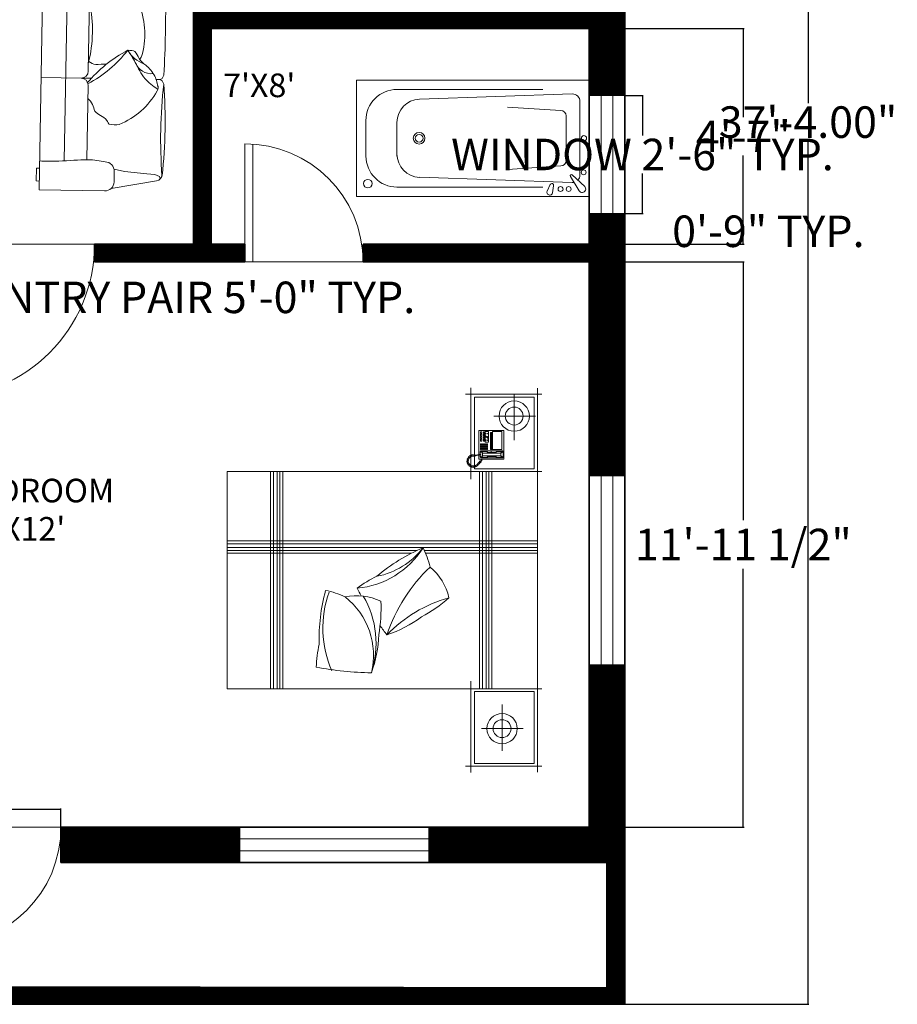
# Model space of a CAD drawing. Units: inches. Extents: x 108 to 771, y 58 to 590.
# Tile 7 of 8: x 524 to 747, y 100 to 350. Entities that reach past the tile are written whole.
import ezdxf

# ---------------------------------------------------------------- set-up
doc = ezdxf.new("R2010")
doc.units = ezdxf.units.IN
doc.header["$MEASUREMENT"] = 0
for name, color, linetype, lineweight in [('A-ANNO-DIMS', 2, 'Continuous', 13), ('A-AREA-IDEN', 7, 'Continuous', 18), ('A-DOOR', 3, 'Continuous', 18), ('A-FLOR-FIXT', 8, 'Continuous', 15), ('A-GLAZ', 4, 'Continuous', 18), ('A-WALL', 7, 'Continuous', 35), ('A-WALL-PATT', 252, 'Continuous', 9), ('Furniture', 7, 'Continuous', 15)]:
    doc.layers.add(name, color=color, linetype=linetype, lineweight=lineweight)
doc.styles.get("Standard").update_dxf_attribs({"font": 'italic8.shx'})
doc.dimstyles.get("Standard").update_dxf_attribs({"dimtxt": 8, "dimasz": 0.18, "dimexe": 0.18, "dimexo": 0.0625, "dimgap": 0.09, "dimtad": 0, "dimtih": 1, "dimtoh": 1, "dimzin": 0, "dimdsep": 46, "dimlunit": 3, "dimtxsty": 'Standard', "dimcen": 0.09, "dimclrt": 6, "dimadec": 0, "dimazin": 0, "dimtfac": 1, "dimtofl": 0, "dimtmove": 0, "dimatfit": 3, "dimfxl": 1, "dimtolj": 1, "dimtzin": 0, "dimarcsym": 0})

# ---------------------------------------------------------------- blocks, each defined once
blk = doc.blocks.new('*D6')
at = {"layer": 'A-ANNO-DIMS', "color": 0, "lineweight": -2, "transparency": 16777216}
for p, q in [((677.41, 548.05), (724.06, 548.05)), ((723.88, 547.87), (723.88, 328.9)), ((723.88, 100.23), (723.88, 319.2)), ((677.41, 100.05), (724.06, 100.05))]:
    blk.add_line(p, q, dxfattribs=at)
at = {"layer": 'A-ANNO-DIMS', "color": 0, "transparency": 16777216}
for points in [[(723.85, 547.87), (723.91, 547.87), (723.88, 548.05)], [(723.85, 100.23), (723.91, 100.23), (723.88, 100.05)]]:
    blk.add_solid(points, dxfattribs=at)
at = {"layer": 'Defpoints', "color": 0, "transparency": 16777216}
for p in [(677.35, 548.05), (677.35, 100.05), (723.88, 100.05)]:
    blk.add_point(p, dxfattribs=at)
at = {"layer": 'A-ANNO-DIMS', "color": 0, "transparency": 16777216, "insert": (723.88, 324.05), "char_height": 8, "attachment_point": 5}
blk.add_mtext('\\A1;37\'-4.00"', dxfattribs=at)
blk = doc.blocks.new('DOOR-SINGLE-39')
for p, q in [((0, 39), (0, 0)), ((2, 38.95), (2, 0)), ((0, 0), (39, 0))]:
    blk.add_line(p, q)
blk.add_arc((0, 0), 39, 0, 90)
blk = doc.blocks.new('DOOR-SINGLE-30')
for p, q in [((30, 30), (30, 0)), ((28, 29.93), (28, 0)), ((30, 0), (0, 0))]:
    blk.add_line(p, q)
blk.add_arc((30, 0), 30, 90, 180)
blk = doc.blocks.new('WINDOW-48')
for p, q in [((0, 48), (0, 0)), ((9, 48), (0, 48)), ((3, 48), (3, 0)), ((6, 48), (6, 0)), ((9, 0), (9, 48)), ((0, 0), (9, 0))]:
    blk.add_line(p, q)
blk = doc.blocks.new('WINDOW-30')
for p, q in [((0, 0), (0, 30)), ((0, 30), (9, 30)), ((3, 30), (3, 0)), ((6, 30), (6, 0)), ((9, 30), (9, 0)), ((9, 0), (0, 0))]:
    blk.add_line(p, q)
blk = doc.blocks.new('BATHTUB')
for p, q in [((59.06, 29.53), (0, 29.53)), ((0, 29.53), (0, 0)), ((4.78, 24.45), (2.59, 28.08)), ((9.35, 28.65), (9.04, 26.82)), ((9.94, 26.54), (10.7, 28.16)), ((59.06, 0), (59.06, 29.53)), ((1.15, 27.02), (4.3, 24.06)), ((4.33, 26.04), (43.12, 24.68)), ((48.82, 27.17), (11.81, 27.17)), ((2.36, 24.07), (2.36, 5.46)), ((7.23, 21.79), (20.76, 22.69)), ((5.85, 20.41), (5.85, 9.11)), ((48.82, 10.75), (48.82, 19.29)), ((56.69, 10.24), (56.69, 19.29)), ((7.23, 7.74), (20.76, 6.84)), ((4.33, 3.49), (43.12, 4.85)), ((0, 0), (59.06, 0)), ((11.81, 2.36), (48.82, 2.36))]:
    blk.add_line(p, q)
for centre, radius in [((5.23, 27.66), 0.628), ((7.29, 27.66), 0.628), ((56.21, 26.29), 1.09), ((1.42, 23.41), 0.628), ((1.34, 14.76), 0.656), ((43.18, 14.76), 1.48), ((43.18, 14.76), 0.984)]:
    blk.add_circle(centre, radius)
for centre, radius, start, end in [((1.81, 27.63), 0.903, 29.9808, 223.0225), ((10.05, 28.48), 0.722, 333.7022, 166.7439), ((4.33, 24.07), 1.97, 137.6863, 180), ((4.33, 24.07), 1.97, 137.6863, 180), ((4.33, 24.07), 1.97, 90, 103.842), ((4.33, 24.07), 1.97, 90, 103.842), ((9.51, 26.74), 0.472, 170.4963, 334.8002), ((48.82, 19.29), 7.87, 0, 90), ((4.51, 24.29), 0.315, 226.7749, 31.0788), ((4.51, 24.29), 0.315, 226.7749, 31.0788), ((42.91, 18.78), 5.91, 0, 87.9984), ((7.23, 20.41), 1.38, 90, 180), ((42.91, 10.75), 5.91, 272.0016, 0), ((48.82, 10.24), 7.87, 270, 0), ((7.23, 9.11), 1.38, 180, 270), ((4.33, 5.46), 1.97, 180, 270)]:
    blk.add_arc(centre, radius, start, end)
blk = doc.blocks.new('SOFA')
for p, q in [((13.53, 80.95), (2.06, 78.82)), ((31.83, 81.57, 13.5), (15.2, 81.57, 13.5)), ((31.83, 81.57, 13.5), (31.83, 0)), ((1.33, 77.65), (1.12, 78.32)), ((2.53, 77.19), (1.33, 77.65)), ((12.83, 79.28), (12.82, 76.57)), ((31.83, 79.37, 0.36), (32.62, 79.37, 0.36)), ((32.62, 79.37, 0.36), (32.62, 76.1, 0.36)), ((4.58, 77.03), (2.53, 77.19)), ((10.24, 76.55), (4.58, 77.03)), ((12.88, 76.04), (10.24, 76.55)), ((32.62, 76.1, 0.36), (31.83, 76.1, 0.91)), ((19.88, 73.73), (19.88, 54.83)), ((25.57, 7.53, 9.89), (25.57, 74.14, 9.89)), ((1.09, 53.34), (0.67, 54.21)), ((1.09, 52.77), (0.68, 51.91)), ((1.64, 53.06), (1.09, 53.34)), ((1.64, 53.06), (1.09, 52.77)), ((1.64, 53.06), (2.64, 53.06)), ((19.09, 53.06), (21.65, 53.06)), ((21.65, 53.06), (31.83, 53.06)), ((19.88, 51.29), (19.88, 31.21)), ((1.05, 29.87), (0.64, 30.74)), ((1.19, 29.01), (0.68, 28.32)), ((1.8, 29.44), (1.05, 29.87)), ((1.81, 29.44), (1.19, 29.01)), ((26.18, 29.43), (1.8, 29.43)), ((19.88, 27.66), (19.89, 7.88, 0.34)), ((31.83, 29.43), (21.65, 29.43)), ((2.53, 5.3), (1.33, 4.84)), ((10.24, 5.94), (2.53, 5.3)), ((13.2, 6.51), (10.24, 5.94)), ((12.69, 2.37), (12.69, 5.08)), ((32.62, 5.47, 0.36), (31.83, 5.47, 0.91)), ((32.62, 2.2, 0.36), (32.62, 5.47, 0.36)), ((0.97, 3.69), (0.62, 4.84)), ((1.33, 4.84), (0.97, 3.69)), ((2.18, 3.23), (0.97, 3.69)), ((4.22, 3.07), (2.18, 3.23)), ((9.88, 2.59), (4.22, 3.07)), ((12.84, 2.01), (9.88, 2.59)), ((15.05, 0.01), (31.83, 0)), ((31.83, 2.2, 0.36), (32.62, 2.2, 0.36))]:
    blk.add_line(p, q)
for centre, radius, start, end in [((15.09, 79.31, 13.5), 2.25, 87.0581, 180.9206), ((2.39, 77.08), 1.77, 100.5091, 180), ((123.26, 65.95), 123.14, 174.6632, 185.4698), ((-121.91, 65.95), 123.14, 354.5302, 5.3368), ((15.19, 76.56), 2.36, 179.7859, 269.7859), ((19.84, 46.39, 13.5), 19.99, 113.7986, 151.3924), ((12.86, 58.3, 13.5), 6.47, 76.1804, 99.6612), ((3.85, 55.11, 13.5), 1.77, 151.3924, 203.2188), ((36.72, 25.19, 13.5), 33.78, 119.8342, 142.4564), ((-6.19, 75.47, 13.5), 33.78, 298.4934, 321.1155), ((21.65, 54.83), 1.77, 180, 270), ((21.65, 51.29), 1.77, 90, 180), ((315.61, 40.74), 315.13, 177.9678, 181.8181), ((3.98, 47.34, 13.5), 4.27, 21.4614, 98.0497), ((3.65, 42.24, 13.5), 7.21, 29.4203, 72.7126), ((12.07, 44.11, 13.5), 6.47, 142.7695, 150.2454), ((52.79, 41.52, 13.5), 33.78, 166.9593, 193.0407), ((25.7, 41.94, 13.5), 19.99, 164.3829, 201.9767), ((8.8, 35.12, 13.5), 1.77, 201.9767, 253.8031), ((14.9, 30.29, 13.5), 4.27, 72.0456, 148.634), ((18.62, 26.79, 13.5), 7.21, 80.0046, 123.2969), ((21.65, 31.21), 1.77, 180, 270), ((107.05, 16.32), 107.05, 173.5605, 186.1533), ((24, 18.21, 13.5), 19.99, 151.3169, 188.9106), ((11.21, 23.4, 13.5), 6.47, 113.6986, 137.1794), ((21.65, 27.66), 1.77, 90, 180), ((-18.44, 27.22, 13.5), 38.25, 336.0331, 358.4688), ((50.29, 11.67, 13.5), 33.78, 154.5272, 179.9746), ((6, 15.39, 13.5), 1.77, 188.9106, 240.7371), ((10.84, 9.3, 13.5), 4.27, 58.9796, 135.568), ((13.68, 5.05, 13.5), 7.21, 66.9386, 110.2309), ((15.05, 5.08), 2.36, 90, 180), ((15.05, 2.37), 2.36, 180, 269.9816)]:
    blk.add_arc(centre, radius, start, end)
for points, knots in [([(15.18, 74.2), (16.54, 73.96, 2.2), (19.42, 73.44, 6.84), (25.93, 74.31, 10.25), (30.21, 74.29, 11.73), (31.83, 74.28, 12.29)], [0, 0, 0, 0, 7.670782, 16.13452, 21.306634, 21.306634, 21.306634, 21.306634]), ([(14.41, 64.59, 13.5), (14.41, 64.59, 13.5), (15.3, 62.57, 13.5), (18.13, 62.25, 13.5), (18.49, 59.48, 13.5), (19.41, 58.61, 13.5), (19.88, 58.17, 13.5)], [27.786417, 27.786417, 27.786417, 27.786417, 60.334214, 153.42843, 198.910048, 250.027656, 250.027656, 250.027656, 250.027656]), ([(2.08, 55.2, 13.5), (2.3, 54.16, 13.5), (2.79, 51.93, 13.5), (4.99, 49.65, 13.5), (7.18, 48.12, 13.5), (7.83, 45.76, 13.5), (9.25, 45.77, 13.5), (9.93, 45.78, 13.5)], [0, 0, 0, 0, 3.139621, 6.721226, 9.134784, 11.147372, 12.969489, 12.969489, 12.969489, 12.969489]), ([(2.23, 55.48, 13.5), (3.39, 54.7, 13.5), (5.91, 53.01, 13.5), (7.71, 49.11, 13.5), (9.26, 46.77, 13.5), (9.93, 45.78, 13.5)], [0, 0, 0, 0, 4.104513, 8.93575, 12.539242, 12.539242, 12.539242, 12.539242]), ([(15.26, 49.37, 13.5), (16.21, 49.3, 13.5), (17.85, 49.84, 13.5), (19.2, 49.22, 13.5), (19.79, 48.78, 13.5)], [214.332348, 214.332348, 214.332348, 214.332348, 289.238615, 341.466319, 341.466319, 341.466319, 341.466319]), ([(7.49, 34.11, 13.5), (8.83, 34.51, 13.5), (11.73, 35.38, 13.5), (15.9, 34.29, 13.5), (18.69, 34.01, 13.5), (19.88, 33.9, 13.5)], [0, 0, 0, 0, 4.104513, 8.93575, 12.539242, 12.539242, 12.539242, 12.539242]), ([(7.62, 33.81, 13.5), (8.56, 33.33, 13.5), (10.59, 32.29, 13.5), (13.75, 32.54, 13.5), (16.32, 33.26, 13.5), (18.56, 32.26, 13.5), (19.45, 33.37, 13.5), (19.88, 33.9, 13.5)], [0, 0, 0, 0, 3.139621, 6.721226, 9.134784, 11.147372, 12.969489, 12.969489, 12.969489, 12.969489]), ([(8.61, 29.33, 13.5), (8.61, 29.33, 13.5), (10.55, 28.27, 13.5), (12.98, 29.74, 13.5), (15.37, 27.37, 13.5), (18, 27.79, 13.5), (19.32, 26.76, 13.5), (19.79, 26.2, 13.5)], [27.786417, 27.786417, 27.786417, 27.786417, 60.334214, 153.42843, 198.910048, 289.238615, 341.466319, 341.466319, 341.466319, 341.466319]), ([(4.5, 14.7, 13.5), (5.89, 14.78, 13.5), (8.91, 14.98, 13.5), (12.72, 12.97, 13.5), (15.38, 12.07, 13.5), (16.51, 11.69, 13.5)], [0, 0, 0, 0, 4.104513, 8.93575, 12.539242, 12.539242, 12.539242, 12.539242]), ([(4.55, 14.37, 13.5), (5.36, 13.69, 13.5), (7.1, 12.22, 13.5), (10.24, 11.75, 13.5), (12.91, 11.87, 13.5), (14.86, 10.39, 13.5), (15.98, 11.27, 13.5), (16.51, 11.69, 13.5)], [0, 0, 0, 0, 3.139621, 6.721226, 9.134784, 11.147372, 12.969489, 12.969489, 12.969489, 12.969489]), ([(15.18, 7.47), (16.54, 7.71, 2.2), (19.42, 8.23, 6.84), (25.93, 7.36, 10.25), (30.21, 7.38, 11.73), (31.83, 7.39, 12.29)], [0, 0, 0, 0, 7.670782, 16.13452, 21.306634, 21.306634, 21.306634, 21.306634])]:
    blk.add_open_spline(points, degree=3, knots=knots)
blk = doc.blocks.new('*D22')
at = {"layer": 'A-ANNO-DIMS', "color": 0, "lineweight": -2, "transparency": 16777216}
for p, q in [((677.41, 330.83), (682.03, 330.83)), ((681.85, 330.65), (681.85, 320.68)), ((681.85, 301.01), (681.85, 310.98)), ((677.41, 300.83), (682.03, 300.83))]:
    blk.add_line(p, q, dxfattribs=at)
at = {"layer": 'A-ANNO-DIMS', "color": 0, "transparency": 16777216}
for points in [[(681.82, 330.65), (681.88, 330.65), (681.85, 330.83)], [(681.82, 301.01), (681.88, 301.01), (681.85, 300.83)]]:
    blk.add_solid(points, dxfattribs=at)
at = {"layer": 'Defpoints', "color": 0, "transparency": 16777216}
for p in [(677.35, 330.83), (681.85, 330.83), (677.35, 300.83)]:
    blk.add_point(p, dxfattribs=at)
at = {"layer": 'A-ANNO-DIMS', "color": 6, "transparency": 16777216, "insert": (681.85, 315.83), "char_height": 8, "attachment_point": 5}
blk.add_mtext('\\A1;WINDOW 2\'-6" TYP.', dxfattribs=at)
blk = doc.blocks.new('*D23')
at = {"layer": 'A-ANNO-DIMS', "color": 0, "lineweight": -2, "transparency": 16777216}
for p, q in [((668.35, 300.77), (668.35, 296.15)), ((677.35, 300.77), (677.35, 296.15)), ((668.53, 296.33), (677.17, 296.33)), ((677.35, 296.33), (677.53, 296.33))]:
    blk.add_line(p, q, dxfattribs=at)
at = {"layer": 'A-ANNO-DIMS', "color": 0, "transparency": 16777216}
for points in [[(668.53, 296.36), (668.53, 296.3), (668.35, 296.33)], [(677.17, 296.36), (677.17, 296.3), (677.35, 296.33)]]:
    blk.add_solid(points, dxfattribs=at)
at = {"layer": 'Defpoints', "color": 0, "transparency": 16777216}
for p in [(668.35, 300.83), (677.35, 300.83), (677.35, 296.33)]:
    blk.add_point(p, dxfattribs=at)
at = {"layer": 'A-ANNO-DIMS', "color": 6, "transparency": 16777216, "insert": (713.81, 296.33), "char_height": 8, "attachment_point": 5}
blk.add_mtext('\\A1;0\'-9" TYP.', dxfattribs=at)
blk = doc.blocks.new('*D24')
at = {"layer": 'A-ANNO-DIMS', "color": 0, "lineweight": -2, "transparency": 16777216}
for p, q in [((504.24, 149.55), (504.06, 149.55)), ((504.24, 145.12), (504.24, 149.73)), ((534.06, 149.55), (504.42, 149.55)), ((534.24, 145.12), (534.24, 149.73))]:
    blk.add_line(p, q, dxfattribs=at)
at = {"layer": 'A-ANNO-DIMS', "color": 0, "transparency": 16777216}
for points in [[(504.42, 149.58), (504.42, 149.52), (504.24, 149.55)], [(534.06, 149.58), (534.06, 149.52), (534.24, 149.55)]]:
    blk.add_solid(points, dxfattribs=at)
at = {"layer": 'Defpoints', "color": 0, "transparency": 16777216}
for p in [(504.24, 149.55), (504.24, 145.05), (534.24, 145.05)]:
    blk.add_point(p, dxfattribs=at)
at = {"layer": 'A-ANNO-DIMS', "color": 6, "transparency": 16777216, "insert": (418.64, 149.55), "char_height": 8, "attachment_point": 5}
blk.add_mtext('\\A1;SINGLE DOOR 2\'-6" TYP.', dxfattribs=at)
blk = doc.blocks.new('*D30')
at = {"layer": 'A-ANNO-DIMS', "color": 0, "lineweight": -2, "transparency": 16777216}
for p, q in [((426.12, 288.49), (426.12, 279.37)), ((486.12, 288.49), (486.12, 279.37)), ((426.3, 279.55), (485.94, 279.55)), ((486.12, 279.55), (486.3, 279.55))]:
    blk.add_line(p, q, dxfattribs=at)
at = {"layer": 'A-ANNO-DIMS', "color": 0, "transparency": 16777216}
for points in [[(426.3, 279.58), (426.3, 279.52), (426.12, 279.55)], [(485.94, 279.58), (485.94, 279.52), (486.12, 279.55)]]:
    blk.add_solid(points, dxfattribs=at)
at = {"layer": 'Defpoints', "color": 0, "transparency": 16777216}
for p in [(426.12, 288.55), (486.12, 288.55), (486.12, 279.55)]:
    blk.add_point(p, dxfattribs=at)
at = {"layer": 'A-ANNO-DIMS', "color": 6, "transparency": 16777216, "insert": (568.68, 279.55), "char_height": 8, "attachment_point": 5}
blk.add_mtext('\\A1;ENTRY PAIR 5\'-0" TYP.', dxfattribs=at)
blk = doc.blocks.new('*D49')
at = {"layer": 'A-ANNO-DIMS', "color": 0, "lineweight": -2, "transparency": 16777216}
for p, q in [((668.41, 288.55), (707.63, 288.55)), ((707.45, 288.37), (707.45, 222.99)), ((707.45, 145.23), (707.45, 210.62)), ((668.41, 145.05), (707.63, 145.05))]:
    blk.add_line(p, q, dxfattribs=at)
at = {"layer": 'A-ANNO-DIMS', "color": 0, "transparency": 16777216}
for points in [[(707.42, 288.37), (707.48, 288.37), (707.45, 288.55)], [(707.42, 145.23), (707.48, 145.23), (707.45, 145.05)]]:
    blk.add_solid(points, dxfattribs=at)
at = {"layer": 'Defpoints', "color": 0, "transparency": 16777216}
for p in [(668.35, 288.55), (707.45, 288.55), (668.35, 145.05)]:
    blk.add_point(p, dxfattribs=at)
at = {"layer": 'A-ANNO-DIMS', "color": 6, "transparency": 16777216, "insert": (707.45, 216.8), "char_height": 8, "attachment_point": 5}
blk.add_mtext('\\A1;11\'-11 1/2"', dxfattribs=at)
blk = doc.blocks.new('*D50')
at = {"layer": 'A-ANNO-DIMS', "color": 0, "lineweight": -2, "transparency": 16777216}
for p, q in [((668.41, 347.8), (707.63, 347.8)), ((707.45, 347.62), (707.45, 325.28)), ((707.45, 293.23), (707.45, 315.58)), ((668.41, 293.05), (707.63, 293.05))]:
    blk.add_line(p, q, dxfattribs=at)
at = {"layer": 'A-ANNO-DIMS', "color": 0, "transparency": 16777216}
for points in [[(707.42, 347.62), (707.48, 347.62), (707.45, 347.8)], [(707.42, 293.23), (707.48, 293.23), (707.45, 293.05)]]:
    blk.add_solid(points, dxfattribs=at)
at = {"layer": 'Defpoints', "color": 0, "transparency": 16777216}
for p in [(668.35, 347.8), (707.45, 347.8), (668.35, 293.05)]:
    blk.add_point(p, dxfattribs=at)
at = {"layer": 'A-ANNO-DIMS', "color": 6, "transparency": 16777216, "insert": (707.45, 320.43), "char_height": 8, "attachment_point": 5}
blk.add_mtext('\\A1;4\'-7"', dxfattribs=at)

msp = doc.modelspace()

# ---------------------------------------------------------------- hatches: boundary and pattern name
at = {"layer": 'A-WALL-PATT'}
h = msp.add_hatch(dxfattribs=at)
h.set_pattern_fill('ANSI31', color=256)
h.paths.add_polyline_path([(171.345, 461.548), (162.345, 461.548), (162.345, 390.901), (171.345, 390.901), (171.345, 393.51), (171.345, 402.553), (233.142, 402.553), (233.142, 407.053), (171.345, 407.053)])
h.paths.add_polyline_path([(331.845, 438.553), (336.68, 438.554), (336.68, 443.053), (331.845, 443.053), (331.845, 539.053), (365.02, 539.053), (365.02, 548.053), (280.772, 548.053), (280.772, 539.053), (327.345, 539.053), (327.345, 407.053), (325.63, 407.053), (325.63, 402.553), (331.845, 402.553)])
h.paths.add_polyline_path([(286.63, 407.053), (263.142, 407.053), (263.142, 402.553), (267.345, 402.553), (267.345, 352.303), (171.345, 352.303), (171.345, 360.901), (162.345, 360.901), (162.345, 336.026), (171.345, 336.026), (171.345, 347.803), (267.345, 347.803), (267.345, 293.053), (263.142, 293.053), (263.142, 288.553), (293.037, 288.553), (293.037, 293.053), (271.845, 293.053), (271.845, 402.553), (286.63, 402.553)])
h.paths.add_polyline_path([(466.018, 443.053), (424.345, 443.053), (424.345, 539.053), (453.584, 539.053), (453.584, 548.053), (395.02, 548.053), (395.02, 539.053), (419.845, 539.053), (420.71, 443.053), (372.68, 443.053), (372.68, 438.557), (420.751, 438.561), (421.075, 402.553), (422.061, 293.053), (419.994, 293.053), (419.994, 288.553), (426.124, 288.553), (426.124, 293.053), (424.345, 293.053), (424.345, 402.553), (424.345, 438.553), (466.018, 438.553)])
h.paths.add_polyline_path([(512.345, 539.053), (583.918, 539.053), (583.918, 548.053), (483.584, 548.053), (483.584, 539.053), (507.845, 539.053), (507.845, 443.053), (502.018, 443.053), (502.018, 438.553), (507.845, 438.553), (507.845, 402.553), (515.658, 402.553), (515.658, 407.053), (512.345, 407.053)])
h.paths.add_polyline_path([(232.772, 548.053), (162.345, 548.053), (162.345, 509.548), (171.345, 509.548), (171.345, 539.053), (232.772, 539.053)])
h.paths.add_polyline_path([(233.142, 293.053), (171.345, 293.053), (171.345, 306.026), (162.345, 306.026), (162.345, 230.8), (171.345, 230.8), (171.345, 288.553), (233.142, 288.553)])
h.paths.add_polyline_path([(359.994, 293.053), (332.037, 293.053), (332.037, 288.553), (339.345, 288.553), (339.345, 145.053), (334.469, 145.053), (334.469, 136.053), (339.345, 136.053), (339.345, 104.553), (166.845, 104.553), (166.845, 136.053), (211.837, 136.053), (211.837, 145.053), (171.345, 145.053), (171.345, 182.8), (162.345, 182.8), (162.345, 100.053), (343.845, 100.053), (343.845, 136.053), (400.886, 136.053), (400.886, 145.053), (348.345, 145.053), (348.345, 288.553), (359.994, 288.553)])
h.paths.add_polyline_path([(500.345, 288.553), (503.755, 288.553), (503.755, 293.053), (486.124, 293.053), (486.124, 288.553), (491.345, 288.553), (491.345, 145.053), (448.886, 145.053), (448.886, 136.053), (495.845, 136.053), (495.845, 100.053), (677.345, 100.053), (677.345, 186.265), (668.345, 186.265), (668.345, 145.053), (627.637, 145.053), (627.637, 136.053), (672.845, 136.053), (672.845, 104.278), (500.345, 104.539), (500.345, 136.053), (504.239, 136.053), (504.239, 145.053), (500.345, 145.053)])
h.paths.add_polyline_path([(580.913, 293.053), (572.345, 293.053), (572.345, 347.803), (668.345, 347.803), (668.345, 330.831), (677.345, 330.831), (677.345, 366.853), (668.345, 366.853), (668.345, 352.303), (572.345, 352.303), (572.345, 402.553), (580.418, 402.553), (580.418, 407.053), (554.658, 407.053), (554.658, 402.553), (567.845, 402.553), (567.845, 293.053), (542.755, 293.053), (542.755, 288.553), (580.913, 288.553)])
h.paths.add_polyline_path([(677.345, 300.831), (668.345, 300.831), (668.345, 293.053), (610.913, 293.053), (610.913, 288.553), (668.345, 288.553), (668.345, 234.265), (677.345, 234.265)])
h.paths.add_polyline_path([(304.469, 145.053), (259.837, 145.053), (259.837, 136.053), (304.469, 136.053)], flags=17)
h.paths.add_polyline_path([(579.637, 145.053), (534.239, 145.053), (534.239, 136.053), (579.637, 136.053)], flags=17)
h.paths.add_polyline_path([(677.345, 450.416), (668.345, 450.416), (668.345, 407.053), (610.418, 407.053), (610.418, 402.553), (668.345, 402.553), (668.345, 396.853), (677.345, 396.853)])
h.paths.add_polyline_path([(677.345, 548.053), (631.918, 548.053), (631.918, 539.053), (668.345, 539.053), (668.345, 498.416), (677.345, 498.416)])
h = msp.add_hatch(dxfattribs=at)
h.set_pattern_fill('ANSI31', color=256)
h.paths.add_polyline_path([(365.02, 548.053), (280.772, 548.053), (280.772, 539.053), (327.345, 539.053), (327.345, 407.053), (325.63, 407.053), (325.63, 402.553), (331.845, 402.553), (331.845, 438.553), (336.68, 438.554), (336.68, 443.053), (331.845, 443.053), (331.845, 539.053), (365.02, 539.053)])
h.paths.add_polyline_path([(453.584, 548.053), (395.02, 548.053), (395.02, 539.053), (419.845, 539.053), (420.71, 443.053), (372.68, 443.053), (372.68, 438.557), (420.751, 438.561), (421.075, 402.553), (422.061, 293.053), (419.994, 293.053), (419.994, 288.553), (426.124, 288.553), (426.124, 293.053), (424.345, 293.053), (424.345, 402.553), (424.345, 438.553), (466.018, 438.553), (466.018, 443.053), (424.345, 443.053), (424.345, 539.053), (453.584, 539.053)])
h.paths.add_polyline_path([(232.772, 548.053), (162.345, 548.053), (162.345, 509.548), (171.345, 509.548), (171.345, 539.053), (232.772, 539.053)])
h.paths.add_polyline_path([(171.345, 461.548), (162.345, 461.548), (162.345, 390.901), (171.345, 390.901), (171.345, 393.51), (171.345, 402.553), (233.142, 402.553), (233.142, 407.053), (171.345, 407.053)])
h.paths.add_polyline_path([(286.63, 407.053), (263.142, 407.053), (263.142, 402.553), (267.345, 402.553), (267.345, 352.303), (171.345, 352.303), (171.345, 360.901), (162.345, 360.901), (162.345, 336.026), (171.345, 336.026), (171.345, 347.803), (267.345, 347.803), (267.345, 293.053), (263.142, 293.053), (263.142, 288.553), (293.037, 288.553), (293.037, 293.053), (271.845, 293.053), (271.845, 402.553), (286.63, 402.553)])
h.paths.add_polyline_path([(171.345, 306.026), (162.345, 306.026), (162.345, 230.8), (171.345, 230.8), (171.345, 288.553), (233.142, 288.553), (233.142, 293.053), (171.345, 293.053)])
h.paths.add_polyline_path([(348.345, 288.553), (359.994, 288.553), (359.994, 293.053), (332.037, 293.053), (332.037, 288.553), (339.345, 288.553), (339.345, 145.053), (334.469, 145.053), (334.469, 136.053), (339.345, 136.053), (339.345, 104.553), (166.845, 104.553), (166.845, 136.053), (211.837, 136.053), (211.837, 145.053), (171.345, 145.053), (171.345, 182.8), (162.345, 182.8), (162.345, 100.053), (343.845, 100.053), (343.845, 136.053), (400.886, 136.053), (400.886, 145.053), (348.345, 145.053)])
h.paths.add_polyline_path([(503.755, 293.053), (486.124, 293.053), (486.124, 288.553), (491.345, 288.553), (491.345, 145.053), (448.886, 145.053), (448.886, 136.053), (495.845, 136.053), (495.845, 100.053), (677.345, 100.053), (677.345, 186.265), (668.345, 186.265), (668.345, 145.053), (627.637, 145.053), (627.637, 136.053), (672.845, 136.053), (672.845, 104.278), (500.345, 104.539), (500.345, 136.053), (504.239, 136.053), (504.239, 145.053), (500.345, 145.053), (500.345, 288.553), (503.755, 288.553)])
h.paths.add_polyline_path([(580.913, 293.053), (572.345, 293.053), (572.345, 347.803), (668.345, 347.803), (668.345, 330.831), (677.345, 330.831), (677.345, 366.853), (668.345, 366.853), (668.345, 352.303), (572.345, 352.303), (572.345, 402.553), (580.418, 402.553), (580.418, 407.053), (554.658, 407.053), (554.658, 402.553), (567.845, 402.553), (567.845, 293.053), (542.755, 293.053), (542.755, 288.553), (580.913, 288.553)])
h.paths.add_polyline_path([(677.345, 300.831), (668.345, 300.831), (668.345, 293.053), (610.913, 293.053), (610.913, 288.553), (668.345, 288.553), (668.345, 234.265), (677.345, 234.265)])
h.paths.add_polyline_path([(579.637, 145.053), (534.239, 145.053), (534.239, 136.053), (579.637, 136.053)], flags=17)
h.paths.add_polyline_path([(304.469, 145.053), (259.837, 145.053), (259.837, 136.053), (304.469, 136.053)], flags=17)
h.paths.add_polyline_path([(583.918, 548.053), (483.584, 548.053), (483.584, 539.053), (507.845, 539.053), (507.845, 443.053), (502.018, 443.053), (502.018, 438.553), (507.845, 438.553), (507.845, 402.553), (515.658, 402.553), (515.658, 407.053), (512.345, 407.053), (512.345, 539.053), (583.918, 539.053)])
h.paths.add_polyline_path([(677.345, 548.053), (631.918, 548.053), (631.918, 539.053), (668.345, 539.053), (668.345, 498.416), (677.345, 498.416)])
h.paths.add_polyline_path([(677.345, 450.416), (668.345, 450.416), (668.345, 407.053), (610.418, 407.053), (610.418, 402.553), (668.345, 402.553), (668.345, 396.853), (677.345, 396.853)])

# ---------------------------------------------------------------- linework, layer by layer
at = {"layer": 'A-WALL'}
for p, q in [((677.345, 548.053), (677.345, 100.053)), ((567.845, 402.553), (567.845, 293.053)), ((572.345, 347.803), (668.345, 347.803)), ((572.345, 347.803), (572.345, 293.053)), ((668.345, 347.803), (668.345, 293.053)), ((567.845, 293.053), (542.755, 293.053)), ((542.755, 288.553), (542.755, 293.053)), ((580.913, 293.053), (572.345, 293.053)), ((580.913, 288.553), (580.913, 293.053)), ((668.345, 293.053), (610.913, 293.053)), ((610.913, 288.553), (610.913, 293.053)), ((580.913, 288.553), (542.755, 288.553)), ((668.345, 288.553), (610.913, 288.553)), ((668.345, 288.553), (668.345, 145.053)), ((668.345, 145.053), (534.239, 145.053)), ((534.239, 136.053), (534.239, 145.053)), ((672.845, 136.053), (534.239, 136.053)), ((672.845, 136.053), (672.845, 104.278)), ((672.845, 104.278), (500.345, 104.539)), ((677.345, 100.053), (495.845, 100.053))]:
    msp.add_line(p, q, dxfattribs=at)
at = {"layer": 'Furniture'}
for p, q in [((638.277, 256.577), (638.277, 233.351)), ((649.29, 255.054), (649.29, 243.257)), ((655.207, 233.802), (655.207, 256.487)), ((656.325, 254.961), (636.894, 254.961)), ((639.203, 254.24), (639.203, 236.018)), ((654.387, 254.24), (639.203, 254.24)), ((654.387, 236.018), (654.387, 254.24)), ((644.095, 249.412), (654.661, 249.412)), ((640.368, 245.724), (640.278, 245.634)), ((640.278, 239.651), (640.278, 245.634)), ((646.578, 245.724), (640.368, 245.724)), ((640.773, 245.409), (641.043, 245.409)), ((640.773, 244.959), (640.773, 245.409)), ((640.984, 245.409), (641.043, 245.35)), ((641.043, 245.409), (641.043, 244.959)), ((641.538, 245.409), (641.538, 244.959)), ((641.718, 245.409), (641.538, 245.409)), ((641.718, 244.959), (641.718, 245.409)), ((641.943, 245.454), (641.943, 242.799)), ((642.753, 245.454), (641.943, 245.454)), ((642.168, 245.004), (642.033, 245.004)), ((642.033, 245.004), (642.033, 244.869)), ((642.168, 244.869), (642.168, 245.004)), ((642.663, 245.004), (642.528, 245.004)), ((642.528, 245.004), (642.528, 244.869)), ((642.663, 244.869), (642.663, 245.004)), ((642.753, 242.799), (642.753, 245.454)), ((643.248, 245.274), (643.248, 240.954)), ((643.698, 245.274), (643.248, 245.274)), ((643.417, 245.274), (643.417, 240.954)), ((643.698, 240.954), (643.698, 245.274)), ((643.788, 245.454), (643.788, 240.954)), ((646.173, 245.454), (643.788, 245.454)), ((646.173, 240.954), (646.173, 245.454)), ((646.668, 245.634), (646.578, 245.724)), ((646.668, 245.634), (646.668, 238.524)), ((641.043, 244.959), (640.773, 244.959)), ((640.773, 244.779), (641.043, 244.779)), ((640.773, 244.329), (640.773, 244.779)), ((641.043, 244.329), (640.773, 244.329)), ((640.773, 244.149), (641.043, 244.149)), ((640.773, 243.699), (640.773, 244.149)), ((641.043, 243.699), (640.773, 243.699)), ((640.773, 243.069), (640.773, 243.519)), ((640.773, 243.519), (641.043, 243.519)), ((641.043, 243.069), (640.773, 243.069)), ((641.043, 244.779), (641.043, 244.329)), ((641.043, 244.149), (641.043, 243.699)), ((641.043, 243.519), (641.043, 243.069)), ((641.538, 244.959), (641.718, 244.959)), ((641.538, 244.779), (641.538, 244.329)), ((641.718, 244.779), (641.538, 244.779)), ((641.538, 244.329), (641.718, 244.329)), ((641.538, 244.149), (641.538, 243.699)), ((641.718, 244.149), (641.538, 244.149)), ((641.538, 243.699), (641.718, 243.699)), ((641.718, 243.519), (641.538, 243.519)), ((641.538, 243.519), (641.538, 243.069)), ((641.538, 243.069), (641.718, 243.069)), ((641.614, 244.779), (641.718, 244.675)), ((641.718, 244.329), (641.718, 244.779)), ((641.718, 243.699), (641.718, 244.149)), ((641.718, 243.069), (641.718, 243.519)), ((641.943, 244.45), (642.753, 243.64)), ((641.943, 242.799), (642.753, 242.799)), ((642.033, 244.869), (642.168, 244.869)), ((642.033, 244.194), (642.033, 244.059)), ((642.168, 244.194), (642.033, 244.194)), ((642.033, 244.059), (642.168, 244.059)), ((642.033, 243.384), (642.033, 243.249)), ((642.168, 243.384), (642.033, 243.384)), ((642.033, 243.249), (642.168, 243.249)), ((642.168, 244.059), (642.168, 244.194)), ((642.168, 243.249), (642.168, 243.384)), ((642.528, 244.869), (642.663, 244.869)), ((642.528, 244.194), (642.528, 244.059)), ((642.663, 244.194), (642.528, 244.194)), ((642.528, 244.059), (642.663, 244.059)), ((642.528, 243.384), (642.528, 243.249)), ((642.663, 243.384), (642.528, 243.384)), ((642.528, 243.249), (642.663, 243.249)), ((642.663, 244.059), (642.663, 244.194)), ((642.663, 243.249), (642.663, 243.384)), ((643.698, 244.914), (643.248, 244.914)), ((643.698, 244.554), (643.248, 244.554)), ((643.698, 244.194), (643.248, 244.194)), ((643.698, 243.834), (643.248, 243.834)), ((643.698, 243.474), (643.248, 243.474)), ((643.248, 243.145), (643.417, 242.976)), ((643.698, 243.114), (643.248, 243.114)), ((640.638, 240.324), (640.863, 240.549)), ((640.638, 239.691), (640.638, 240.324)), ((640.683, 240.189), (640.773, 240.369)), ((640.683, 240.189), (640.683, 239.692)), ((641.268, 239.964), (640.683, 240.189)), ((640.728, 242.394), (640.998, 242.394)), ((640.728, 242.034), (640.728, 242.394)), ((640.998, 242.034), (640.728, 242.034)), ((640.728, 241.494), (640.728, 241.854)), ((640.728, 241.854), (640.998, 241.854)), ((640.998, 241.494), (640.728, 241.494)), ((640.728, 241.314), (640.998, 241.314)), ((640.728, 240.954), (640.728, 241.314)), ((640.998, 240.954), (640.728, 240.954)), ((640.773, 240.369), (640.953, 240.414)), ((640.863, 240.549), (646.308, 240.549)), ((640.953, 240.414), (642.168, 240.414)), ((640.953, 240.414), (641.358, 240.009)), ((640.998, 242.394), (640.998, 242.034)), ((640.998, 241.854), (640.998, 241.494)), ((640.998, 241.314), (640.998, 240.954)), ((641.223, 242.394), (641.493, 242.394)), ((641.223, 242.034), (641.223, 242.394)), ((641.493, 242.034), (641.223, 242.034)), ((641.223, 241.854), (641.493, 241.854)), ((641.223, 241.494), (641.223, 241.854)), ((641.493, 241.494), (641.223, 241.494)), ((641.268, 241.314), (641.538, 241.314)), ((641.268, 240.954), (641.268, 241.314)), ((641.538, 240.954), (641.268, 240.954)), ((641.358, 240.009), (641.268, 239.964)), ((643.788, 240.009), (641.358, 240.009)), ((641.493, 242.394), (641.493, 242.034)), ((641.493, 241.854), (641.493, 241.494)), ((641.538, 241.314), (641.538, 240.954)), ((641.763, 242.394), (642.033, 242.394)), ((641.763, 242.034), (641.763, 242.394)), ((642.033, 242.034), (641.763, 242.034)), ((641.763, 241.854), (642.033, 241.854)), ((641.763, 241.494), (641.763, 241.854)), ((642.033, 241.494), (641.763, 241.494)), ((641.763, 241.314), (642.033, 241.314)), ((641.763, 240.954), (641.763, 241.314)), ((642.033, 240.954), (641.763, 240.954)), ((642.033, 242.394), (642.033, 242.034)), ((642.033, 241.854), (642.033, 241.494)), ((642.033, 241.314), (642.033, 240.954)), ((642.168, 240.414), (642.393, 240.324)), ((642.258, 242.394), (642.528, 242.394)), ((642.258, 242.034), (642.258, 242.394)), ((642.528, 242.034), (642.258, 242.034)), ((642.258, 241.854), (642.528, 241.854)), ((642.258, 241.494), (642.258, 241.854)), ((642.528, 241.494), (642.258, 241.494)), ((642.258, 240.954), (642.258, 241.314)), ((642.258, 241.314), (642.528, 241.314)), ((642.528, 240.954), (642.258, 240.954)), ((642.393, 240.324), (642.618, 240.189)), ((642.528, 242.394), (642.528, 242.034)), ((642.528, 241.854), (642.528, 241.494)), ((642.528, 241.314), (642.528, 240.954)), ((642.618, 240.189), (642.933, 240.144)), ((642.933, 240.144), (643.788, 240.144)), ((643.248, 240.954), (643.698, 240.954)), ((643.417, 240.549), (643.417, 240.144)), ((643.788, 240.954), (646.173, 240.954)), ((644.238, 240.144), (643.788, 240.144)), ((643.788, 240.009), (645.813, 240.009)), ((644.553, 240.189), (644.238, 240.144)), ((644.778, 240.324), (644.553, 240.189)), ((645.003, 240.414), (644.778, 240.324)), ((646.218, 240.414), (645.003, 240.414)), ((646.218, 240.414), (645.813, 240.009)), ((645.813, 240.009), (645.903, 239.964)), ((645.903, 239.964), (646.488, 240.189)), ((646.398, 240.369), (646.218, 240.414)), ((646.308, 240.549), (646.533, 240.369)), ((646.488, 240.189), (646.398, 240.369)), ((646.488, 240.189), (646.488, 239.109)), ((646.533, 240.369), (646.533, 239.019)), ((637.56, 237.93), (637.268, 237.83)), ((637.268, 237.83), (637.314, 237.657)), ((637.314, 238.149), (637.295, 237.994)), ((637.295, 237.994), (637.56, 237.93)), ((637.368, 238.567), (637.314, 238.376)), ((637.314, 238.376), (637.56, 238.258)), ((637.56, 238.258), (637.314, 238.149)), ((637.314, 237.657), (637.56, 237.648)), ((637.669, 238.54), (637.368, 238.567)), ((637.56, 237.648), (637.377, 237.438)), ((637.596, 238.932), (637.487, 238.759)), ((637.487, 238.759), (637.669, 238.54)), ((637.842, 238.895), (637.596, 238.932)), ((637.642, 237.793), (637.687, 238.34)), ((637.869, 237.265), (637.642, 237.793)), ((637.851, 239.241), (637.687, 239.105)), ((637.687, 239.105), (637.842, 238.895)), ((637.687, 238.34), (637.942, 238.822)), ((638.106, 239.114), (637.851, 239.241)), ((637.942, 238.822), (638.38, 239.168)), ((638.261, 239.505), (638.052, 239.387)), ((638.052, 239.387), (638.106, 239.114)), ((638.462, 239.25), (638.261, 239.505)), ((638.38, 239.168), (638.954, 239.214)), ((638.489, 239.542), (638.462, 239.25)), ((638.735, 239.56), (638.489, 239.542)), ((638.89, 239.305), (638.735, 239.56)), ((638.936, 239.569), (638.89, 239.305)), ((639.154, 239.551), (638.936, 239.569)), ((638.954, 239.214), (639.163, 239.178)), ((639.254, 239.451), (639.154, 239.551)), ((639.163, 239.178), (639.282, 239.341)), ((639.309, 239.478), (639.254, 239.451)), ((639.282, 239.341), (639.519, 239.332)), ((639.546, 239.469), (639.309, 239.478)), ((639.519, 239.332), (639.737, 239.36)), ((639.974, 239.578), (639.546, 239.469)), ((639.737, 239.36), (640.166, 239.469)), ((640.324, 237.641), (639.817, 237.046)), ((640.43, 239.688), (639.974, 239.578)), ((640.166, 239.469), (640.457, 239.533)), ((640.278, 238.524), (640.278, 239.494)), ((640.368, 238.434), (640.278, 238.524)), ((640.649, 238.005), (640.324, 237.641)), ((646.578, 238.434), (640.368, 238.434)), ((640.538, 237.379), (640.411, 237.625)), ((640.411, 237.625), (640.673, 237.53)), ((640.818, 239.694), (640.43, 239.688)), ((640.457, 239.533), (640.818, 239.559)), ((640.638, 239.019), (640.638, 239.546)), ((640.908, 238.794), (640.638, 239.019)), ((640.745, 237.91), (640.649, 238.005)), ((640.673, 237.53), (640.8, 237.649)), ((640.683, 239.549), (640.683, 239.109)), ((641.268, 239.334), (640.683, 239.109)), ((640.683, 239.109), (640.773, 238.929)), ((640.8, 237.649), (640.713, 237.76)), ((640.713, 237.76), (640.848, 237.696)), ((640.8, 238.053), (640.737, 238.005)), ((640.737, 238.005), (640.745, 237.91)), ((640.773, 238.929), (640.953, 238.884)), ((640.943, 238.235), (640.8, 238.053)), ((640.818, 239.559), (640.818, 239.694)), ((640.848, 237.696), (640.927, 237.775)), ((640.863, 237.942), (640.951, 238.037)), ((640.927, 237.775), (640.863, 237.942)), ((646.308, 238.794), (640.908, 238.794)), ((640.998, 238.434), (640.943, 238.235)), ((640.951, 238.037), (641.078, 238.164)), ((640.953, 238.884), (641.358, 239.289)), ((640.953, 238.884), (642.168, 238.884)), ((641.078, 238.164), (641.178, 238.434)), ((641.268, 239.334), (641.268, 239.964)), ((641.358, 239.289), (641.268, 239.334)), ((643.788, 239.289), (641.358, 239.289)), ((642.168, 238.884), (642.393, 238.974)), ((642.393, 238.974), (642.618, 239.109)), ((642.618, 239.109), (642.933, 239.154)), ((642.933, 239.154), (643.788, 239.154)), ((643.788, 239.289), (645.813, 239.289)), ((644.238, 239.154), (643.788, 239.154)), ((644.553, 239.109), (644.238, 239.154)), ((644.778, 238.974), (644.553, 239.109)), ((645.003, 238.884), (644.778, 238.974)), ((646.218, 238.884), (645.003, 238.884)), ((645.813, 239.289), (645.903, 239.334)), ((646.218, 238.884), (645.813, 239.289)), ((645.903, 239.334), (645.903, 239.964)), ((645.903, 239.334), (646.488, 239.109)), ((646.398, 238.929), (646.218, 238.884)), ((646.533, 239.019), (646.308, 238.794)), ((646.488, 239.109), (646.398, 238.929)), ((646.668, 238.524), (646.578, 238.434)), ((576.467, 235.297), (655.207, 235.297)), ((576.467, 180.179), (576.467, 235.297)), ((587.443, 180.179), (587.443, 235.297)), ((588.199, 180.179), (588.199, 235.297)), ((589.089, 180.179), (589.089, 235.297)), ((589.831, 180.179), (589.831, 235.297)), ((590.573, 180.179), (590.573, 235.297)), ((656.325, 235.297), (636.894, 235.297)), ((637.377, 237.438), (637.45, 237.292)), ((637.45, 237.292), (637.724, 237.32)), ((637.724, 237.32), (637.487, 237.129)), ((637.487, 237.129), (637.614, 236.983)), ((637.614, 236.983), (637.86, 237.092)), ((637.86, 237.092), (637.751, 236.837)), ((637.751, 236.837), (637.86, 236.719)), ((637.86, 236.719), (638.106, 236.846)), ((638.261, 236.864), (637.869, 237.265)), ((638.106, 236.846), (638.024, 236.582)), ((638.024, 236.582), (638.207, 236.509)), ((638.207, 236.509), (638.453, 236.728)), ((638.945, 236.737), (638.261, 236.864)), ((638.417, 236.835), (638.417, 236.696)), ((638.453, 236.728), (638.443, 236.446)), ((638.443, 236.446), (638.626, 236.409)), ((638.626, 236.409), (638.762, 236.646)), ((638.762, 236.646), (638.844, 236.364)), ((638.844, 236.364), (639.072, 236.409)), ((639.801, 237.037), (638.945, 236.737)), ((639.072, 236.409), (639.072, 236.655)), ((639.072, 236.655), (639.254, 236.464)), ((639.203, 236.018), (654.387, 236.018)), ((639.254, 236.464), (639.464, 236.527)), ((639.464, 236.527), (639.455, 236.819)), ((639.455, 236.819), (639.555, 236.555)), ((639.555, 236.555), (639.829, 236.637)), ((639.801, 236.911), (639.999, 236.84)), ((639.829, 236.637), (639.801, 236.91)), ((639.999, 236.84), (640.181, 237.014)), ((640.054, 237.221), (640.34, 237.173)), ((640.181, 237.014), (640.054, 237.221)), ((640.34, 237.173), (640.538, 237.379)), ((640.505, 180.179), (640.505, 235.297)), ((641.261, 180.179), (641.261, 235.297)), ((642.151, 180.179), (642.151, 235.297)), ((642.893, 180.179), (642.893, 235.297)), ((643.635, 180.179), (643.635, 235.297)), ((655.207, 180.179), (655.207, 235.297)), ((576.467, 217.69), (655.207, 217.69)), ((576.467, 216.934), (655.207, 216.934)), ((576.467, 216.044), (655.207, 216.044)), ((576.467, 215.302), (624.672, 215.302)), ((626.475, 215.302), (655.207, 215.302)), ((576.467, 214.56), (623.161, 214.56)), ((626.805, 214.56), (655.207, 214.56)), ((655.207, 180.179), (576.467, 180.179)), ((656.325, 180.179), (636.894, 180.179)), ((638.277, 158.9), (638.277, 182.125)), ((655.207, 181.675), (655.207, 158.99)), ((639.203, 161.236), (639.203, 179.458)), ((639.203, 179.458), (654.387, 179.458)), ((654.387, 179.458), (654.387, 161.236)), ((646.212, 164.403), (646.212, 176.201)), ((641.016, 170.046), (651.582, 170.046)), ((656.325, 160.515), (636.894, 160.515)), ((654.387, 161.236), (639.203, 161.236))]:
    msp.add_line(p, q, dxfattribs=at)
for centre, radius in [((649.29, 249.412), 3.847), ((649.29, 249.412), 2.272), ((646.212, 170.046), 3.847), ((646.212, 170.046), 2.272)]:
    msp.add_circle(centre, radius, dxfattribs=at)
for centre, radius, start, end in [((607.334, 227.864), 22.265, 275.33912, 327.68949), ((644.123, 173.756), 45.873, 113.06416, 130.32086), ((610.874, 227.607), 19.209, 280.69865, 322.68638), ((606.935, 206.156), 21.574, 13.20343, 27.03623), ((657.272, 180.314), 42.512, 133.63057, 161.4288), ((618.978, 200.228), 14.076, 12.47819, 50.46254), ((626.771, 182.596), 28.899, 115.25901, 126.93514), ((645.65, 192.981), 45.873, 164.62778, 181.88448), ((597.154, 183.992), 21.574, 64.76704, 78.59984), ((685.854, 246.215), 86.523, 207.92482, 209.3793), ((627.819, 195.596), 27.107, 160.29361, 203.6414), ((609.284, 189.741), 14.076, 64.0418, 102.02615), ((594.779, 188.696), 18.796, 346.18494, 52.00166), ((590.273, 191.686), 23.956, 341.81005, 30.13512), ((641.778, 170.249), 34.24, 105.33601, 136.41927), ((607.175, 232.599), 38.896, 298.49711, 311.05657), ((576.59, 200.619), 38.896, 350.06073, 2.62018), ((607.214, 223.275), 30.999, 288.35266, 306.68512), ((685.854, 246.215), 86.523, 215.29657, 217.24182), ((583.918, 194.853), 30.999, 339.91627, 358.24873), ((627.94, 184.884), 28.899, 166.82262, 178.49876), ((614.835, 270.712), 86.523, 259.48843, 268.80544)]:
    msp.add_arc(centre, radius, start, end, dxfattribs=at)

# ---------------------------------------------------------------- block references
at = {"layer": 'A-DOOR', "extrusion": (0, 0, -1), "zscale": -1}
msp.add_blockref('DOOR-SINGLE-30', (-610.913, 288.553), dxfattribs=at)
at = {"layer": 'A-DOOR', "extrusion": (0, 0, -1), "zscale": -1, "rotation": 180}
msp.add_blockref('DOOR-SINGLE-39', (-503.755, 293.053), dxfattribs=at)
at = {"layer": 'A-DOOR', "rotation": 180}
msp.add_blockref('DOOR-SINGLE-30', (534.239, 145.053), dxfattribs=at)
at = {"layer": 'A-FLOR-FIXT', "rotation": 180}
msp.add_blockref('BATHTUB', (668.346, 334.713), dxfattribs=at)
at = {"layer": 'A-GLAZ'}
for name, p in [('WINDOW-30', (668.345, 300.831)), ('WINDOW-48', (668.345, 186.265))]:
    msp.add_blockref(name, p, dxfattribs=at)
at = {"layer": 'A-GLAZ', "rotation": 269.9999999999993}
msp.add_blockref('WINDOW-48', (579.637, 145.053), dxfattribs=at)
at = {"layer": 'Furniture', "rotation": 178.9570258815186}
msp.add_blockref('SOFA', (561.991, 387.871), dxfattribs=at)

# ---------------------------------------------------------------- texts
at = {"layer": 'A-AREA-IDEN'}
for s, p in [("7'X8'", (575.409, 330.385)), ('BEDROOM', (507.917, 227.496)), ("12'X12'", (507.917, 217.781))]:
    msp.add_text(s, height=6, dxfattribs=at).set_placement(p)
at = {"layer": 'Furniture', "flags": 9}
for tag, s in [('YSIZE', '806.5825'), ('XSIZE', '855.2549'), ('ZSIZE', '0.0000')]:
    msp.add_attdef(tag, (611.862, 198.974), s, height=0.0197, dxfattribs=at)

# ---------------------------------------------------------------- dimensions: what is measured, and where the dimension line sits
at = {"layer": 'A-ANNO-DIMS'}
for base, p1, p2, override, picture, middle in [((723.88, 100.053), (677.345, 548.053), (677.345, 100.053), {"dimclrd": 0, "dimclre": 0, "dimclrt": 0}, '*D6', (723.88, 324.053)), ((707.445389, 347.803083), (668.345389, 293.053083), (668.345389, 347.803083), {"dimdec": 1, "dimlfac": 1, "dimrnd": 0, "dimzin": 1, "dimdsep": 46, "dimlunit": 4, "dimfrac": 2}, '*D50', (707.445389, 320.428083)), ((707.445, 288.553), (668.345, 145.053), (668.345, 288.553), {"dimdec": 1, "dimlfac": 1, "dimrnd": 0, "dimzin": 1, "dimdsep": 46, "dimlunit": 4, "dimfrac": 2}, '*D49', (707.445, 216.803))]:
    dim = msp.add_linear_dim(base=base, p1=p1, p2=p2, angle=90, dimstyle='Standard', override=override, dxfattribs=at)
    dim.commit()
    dim.dimension.update_dxf_attribs({"geometry": picture, "text_midpoint": middle})
for base, p1, p2, angle, text, picture, middle in [((681.845, 330.831), (677.345, 300.831), (677.345, 330.831), 90, 'WINDOW <> TYP.', '*D22', (681.845, 315.831)), ((504.239, 149.553), (534.239, 145.053), (504.239, 145.053), 180, 'SINGLE DOOR <> TYP.', '*D24', (418.635, 149.553))]:
    dim = msp.add_linear_dim(base=base, p1=p1, p2=p2, angle=angle, text=text, dimstyle='Standard', override={"dimdec": 1, "dimlfac": 1, "dimrnd": 0, "dimzin": 1, "dimdsep": 46, "dimlunit": 4, "dimfrac": 2}, dxfattribs=at)
    dim.commit()
    dim.dimension.update_dxf_attribs({"geometry": picture, "text_midpoint": middle})
for base, p1, p2, text, picture, middle in [((677.345, 296.331), (668.345, 300.831), (677.345, 300.831), '<> TYP.', '*D23', (713.806, 296.331)), ((486.124, 279.553), (426.124, 288.553), (486.124, 288.553), 'ENTRY PAIR <> TYP.', '*D30', (568.679, 279.553))]:
    dim = msp.add_linear_dim(base=base, p1=p1, p2=p2, text=text, dimstyle='Standard', override={"dimdec": 1, "dimlfac": 1, "dimrnd": 0, "dimzin": 1, "dimdsep": 46, "dimlunit": 4, "dimfrac": 2}, dxfattribs=at)
    dim.commit()
    dim.dimension.update_dxf_attribs({"geometry": picture, "text_midpoint": middle})

doc.saveas('drawing.dxf')
